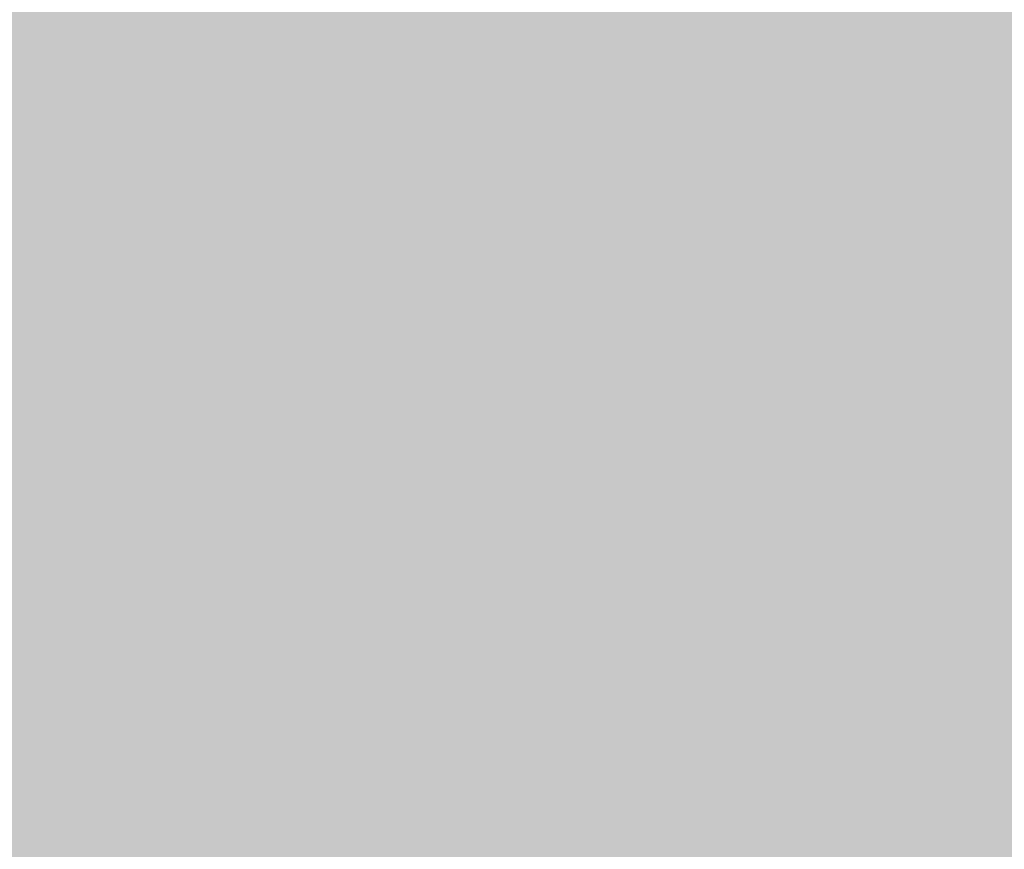
# Model space of a CAD drawing. Units: feet. Extents: x 3168 to 4724, y 827 to 1477.
# Tile 55 of 256: x 3273.13944 to 3273.15625, y 1099.00068 to 1099.01485. Entities that reach past the tile are written whole.
import ezdxf

# ---------------------------------------------------------------- set-up
doc = ezdxf.new("R2010")
doc.units = ezdxf.units.FT
doc.layers.add('A-ELEV', color=7, linetype='Continuous', lineweight=35)
doc.layers.add('A-ELEV-PATT', color=8, linetype='Continuous', lineweight=13)

msp = doc.modelspace()

# ---------------------------------------------------------------- hatches: boundary and pattern name
at = {"layer": 'A-ELEV-PATT'}
h = msp.add_hatch(color=256, dxfattribs=at)
h.dxf.hatch_style = 1
edge = h.paths.add_edge_path()
edge.add_ellipse((3552.905762, 979.220141), major_axis=(36.744924, 0), ratio=0.484848485, start_angle=0, end_angle=360)
edge = h.paths.add_edge_path()
edge.add_ellipse((3559.891637, 929.252282), major_axis=(36.744924, 0), ratio=0.484848485, start_angle=0, end_angle=360)
edge = h.paths.add_edge_path()
edge.add_line((3299.31681, 1198.606081), (3479.916714, 1198.606081))
edge.add_line((3479.916714, 1198.606081), (3479.916714, 1209.86857))
edge.add_spline(control_points=[(3479.916714, 1209.86857), (3464.301157, 1209.86857), (3448.685601, 1209.86857), (3410.949139, 1209.86857), (3388.828234, 1209.86857), (3355.646876, 1209.86857), (3344.586423, 1209.86857), (3327.995745, 1209.86857), (3322.465518, 1209.86857), (3314.170179, 1209.86857), (3311.405066, 1209.86857), (3307.257396, 1209.86857), (3305.874839, 1209.86857), (3303.801005, 1209.86857), (3303.109726, 1209.86857), (3302.072809, 1209.86857), (3301.72717, 1209.86857), (3301.208711, 1209.86857), (3301.035891, 1209.86857), (3300.776662, 1209.86857), (3300.690252, 1209.86857), (3300.560638, 1209.86857), (3300.517433, 1209.86857), (3300.452625, 1209.86857), (3300.431023, 1209.86857), (3300.398619, 1209.86857), (3300.387818, 1209.86857), (3300.366216, 1209.86857), (3300.345676, 1209.86857), (3300.345548, 1209.86857), (3300.345505, 1209.86857), (3300.343304, 1209.86857), (3300.341146, 1209.868571), (3300.337909, 1209.868571), (3300.33683, 1209.868572), (3300.333942, 1209.868573), (3300.332133, 1209.868574), (3300.325515, 1209.868577), (3300.320706, 1209.868581), (3300.310925, 1209.868592), (3300.305952, 1209.868598), (3300.290511, 1209.868623), (3300.280045, 1209.868646), (3300.232425, 1209.868777), (3300.195298, 1209.868954), (3299.951068, 1209.870608), (3299.744824, 1209.874326), (3299.436827, 1209.883257), (3299.334389, 1209.886792), (3299.181079, 1209.89292), (3299.130033, 1209.895099), (3298.652217, 1209.916801), (3298.22946, 1209.945718), (3297.601631, 1210.002367), (3297.393404, 1210.023464), (3297.082652, 1210.058309), (3296.979332, 1210.070458), (3296.292954, 1210.154861), (3295.718148, 1210.243356), (3294.868717, 1210.39885), (3294.5877, 1210.454478), (3294.169341, 1210.543349), (3294.030415, 1210.573878), (3291.707149, 1211.1012), (3289.65359, 1211.813435), (3285.776259, 1213.563988), (3283.95141, 1214.603478), (3280.512159, 1216.98008), (3278.897241, 1218.317592), (3276.379914, 1220.829489), (3275.416042, 1221.917738), (3274.039342, 1223.7077), (3273.581043, 1224.349535), (3273.143228, 1225.016316)], knot_values=[39.119033, 39.119033, 39.119033, 39.119033, 39.286353, 39.286353, 39.523379, 39.523379, 39.641892, 39.641892, 39.701148, 39.701148, 39.730777, 39.730777, 39.745591, 39.745591, 39.752998, 39.752998, 39.756701, 39.756701, 39.758553, 39.758553, 39.759479, 39.759479, 39.759942, 39.759942, 39.760173, 39.760173, 39.760289, 39.760289, 39.760405, 39.760405, 39.760463, 39.760463, 39.763389, 39.763389, 39.764851, 39.764851, 39.767304, 39.767304, 39.773825, 39.773825, 39.78057, 39.78057, 39.79477, 39.79477, 39.845194, 39.845194, 40.126715, 40.126715, 40.267476, 40.267476, 40.337856, 40.337856, 40.927023, 40.927023, 41.221606, 41.221606, 41.368898, 41.368898, 42.202622, 42.202622, 42.619485, 42.619485, 42.827916, 42.827916, 46.118323, 46.118323, 49.408731, 49.408731, 52.699139, 52.699139, 54.927489, 54.927489, 56.104228, 56.104228, 56.104228, 56.104228], weights=[1, 1, 1, 1, 1, 1, 1, 1, 1, 1, 1, 1, 1, 1, 1, 1, 1, 1, 1, 1, 1, 1, 1, 1, 1, 1, 1, 1, 1, 1, 1, 1, 1, 1, 1, 1, 1, 1, 1, 1, 1, 1, 1, 1, 1, 1, 1, 1, 1, 1, 1, 1, 1, 1, 1, 1, 1, 1, 1, 1, 1, 1, 1, 1, 1, 1, 1, 1, 1, 1, 1, 1, 1, 1], degree=3, periodic=0)
edge.add_line((3273.143228, 1225.016316), (3273.143228, 1099.016316))
edge.add_line((3273.143228, 1099.016316), (3299.31681, 1099.016316))
edge.add_line((3299.31681, 1099.016316), (3299.31681, 1198.606081))
edge = h.paths.add_edge_path()
edge.add_line((3304.758443, 1324.15806), (3479.916714, 1324.15806))
edge.add_line((3479.916714, 1324.15806), (3479.916714, 1335.714618))
edge.add_line((3479.916714, 1335.714618), (3269.161628, 1335.714618))
edge.add_spline(control_points=[(3269.161628, 1335.714618), (3264.024231, 1335.714618), (3258.364118, 1328.958189), (3259.264311, 1323.900274)], knot_values=[0, 0, 0, 0, 15.412191, 15.412191, 15.412191, 15.412191], degree=3, periodic=0)
edge.add_line((3259.264311, 1323.900274), (3265.516849, 1288.769135))
edge.add_line((3265.516849, 1288.769135), (3275.265103, 1261.545626))
edge.add_line((3275.265103, 1261.545626), (3304.758443, 1261.545626))
edge.add_line((3304.758443, 1261.545626), (3304.758443, 1324.15806))
h = msp.add_hatch(color=256, dxfattribs=at)
h.dxf.hatch_style = 1
h.paths.add_polyline_path([(3384.525247, 1099.016316), (3335.029168, 1099.016316), (3299.31681, 1099.016316), (3273.143228, 1099.016316), (3217.565364, 1099.016316), (3168.069285, 827.11626), (3335.029168, 827.11626)])

# ---------------------------------------------------------------- linework, layer by layer
at = {"layer": 'A-ELEV'}
msp.add_open_spline([(3808.5202, 1099.016316), (3808.5202, 1141.413235), (3808.5202, 1183.810154), (3808.5202, 1226.635324), (3808.5202, 1227.063576), (3808.5202, 1227.491828), (3811.491871, 1248.994673), (3814.463542, 1270.497518), (3817.46523, 1292.217564), (3817.495247, 1292.434764), (3817.525264, 1292.651964), (3817.572801, 1310.106748), (3817.620339, 1327.561532), (3817.667877, 1345.016316), (3817.667877, 1345.457962), (3817.667877, 1345.899608), (3817.667877, 1346.456047), (3817.667877, 1346.57084), (3817.667877, 1346.752887), (3817.667877, 1346.820142), (3817.667877, 1346.93487), (3817.667877, 1346.982345), (3817.667877, 1347.038587), (3817.667877, 1347.047356), (3817.667877, 1347.073661), (3817.667877, 1347.059303), (3817.667877, 1347.061545), (3817.667876, 1347.062667), (3817.667875, 1347.066031), (3817.667874, 1347.068274), (3817.66787, 1347.075001), (3817.667866, 1347.079486), (3817.667849, 1347.092937), (3817.667833, 1347.101902), (3817.667766, 1347.12879), (3817.667699, 1347.146705), (3817.667432, 1347.200421), (3817.667165, 1347.236192), (3817.6661, 1347.343385), (3817.665038, 1347.414686), (3817.660812, 1347.628095), (3817.656608, 1347.769708), (3817.63997, 1348.192487), (3817.623509, 1348.471586), (3817.559094, 1349.300067), (3817.496121, 1349.840588), (3817.255432, 1351.424156), (3817.026318, 1352.428785), (3816.306871, 1354.888914), (3815.743745, 1356.268727), (3814.463959, 1358.81921), (3813.746413, 1359.990968), (3812.195838, 1362.172343), (3811.362245, 1363.182124), (3809.588836, 1365.069009), (3808.648816, 1365.946105), (3806.654262, 1367.579616), (3805.599702, 1368.336154), (3803.352891, 1369.722327), (3802.160535, 1370.352386), (3799.600813, 1371.453586), (3798.232688, 1371.925481), (3795.280084, 1372.634624), (3793.693148, 1372.872068), (3791.869441, 1372.92648), (3791.740861, 1372.92922), (3791.353371, 1372.934101), (3791.092707, 1372.932901), (3790.304116, 1372.915068), (3789.769543, 1372.884195), (3789.20919, 1372.830236), (3789.190622, 1372.828424), (3789.134892, 1372.822912), (3789.097705, 1372.819137), (3789.048445, 1372.814008), (3789.0364, 1372.812743), (3789.000256, 1372.808918), (3788.976147, 1372.806325), (3788.949405, 1372.803404), (3788.946786, 1372.803118), (3788.942567, 1372.802655), (3788.940967, 1372.80248), (3788.938572, 1372.802217), (3788.937777, 1372.802129), (3788.935391, 1372.801867), (3788.867535, 1372.794402), (3788.756866, 1372.782228), (3788.701532, 1372.776141), (3788.53553, 1372.75788), (3788.424861, 1372.745707), (3788.092856, 1372.709185), (3787.871519, 1372.684837), (3787.207509, 1372.611793), (3786.764835, 1372.563097), (3785.436814, 1372.417009), (3784.551467, 1372.319617), (3781.895425, 1372.027442), (3780.12473, 1371.832658), (3774.812646, 1371.248307), (3771.271256, 1370.858739), (3760.647088, 1369.690037), (3753.56431, 1368.910902), (3732.315973, 1366.573498), (3718.150416, 1365.015228), (3694.006758, 1362.359326), (3684.028657, 1361.261694), (3674.050557, 1360.164062), (3664.600662, 1360.164062), (3655.150767, 1360.164062), (3626.801081, 1360.164062), (3607.901291, 1360.164062), (3551.20192, 1360.164062), (3513.40234, 1360.164062), (3467.725182, 1360.164062), (3459.847604, 1360.164062), (3436.214873, 1360.164062), (3420.459718, 1360.164062), (3373.194255, 1360.164062), (3341.683946, 1360.164062), (3302.848162, 1360.164062), (3295.522686, 1360.164062), (3286.038292, 1360.164062), (3283.879372, 1360.164062), (3277.402613, 1360.164062), (3273.084773, 1360.164062), (3267.732851, 1360.164062), (3266.698768, 1360.164062), (3263.59652, 1360.164062), (3261.528355, 1360.164062), (3259.236943, 1360.164062), (3259.013697, 1360.164062), (3258.343958, 1360.164062), (3257.897466, 1360.164062), (3257.430998, 1360.164062), (3257.411022, 1360.164062), (3257.370573, 1360.164062), (3257.37547, 1360.164062), (3257.374598, 1360.164062), (3257.373937, 1360.164062), (3257.371956, 1360.164062), (3257.370635, 1360.164061), (3257.366673, 1360.16406), (3257.364032, 1360.164059), (3257.356109, 1360.164053), (3257.350828, 1360.164047), (3257.334987, 1360.164023), (3257.32443, 1360.163998), (3257.292769, 1360.163899), (3257.271676, 1360.163799), (3257.208439, 1360.163398), (3257.166337, 1360.162995), (3257.040206, 1360.161388), (3256.956349, 1360.159783), (3256.705504, 1360.153393), (3256.53924, 1360.147036), (3256.04357, 1360.121916), (3255.717296, 1360.097102), (3254.752446, 1360.000481), (3254.127968, 1359.906513), (3252.180067, 1359.525332), (3250.941574, 1359.143991), (3248.670175, 1358.24329), (3247.635739, 1357.723834), (3245.732632, 1356.603471), (3244.863388, 1356.00206), (3243.253108, 1354.742865), (3242.511972, 1354.084731), (3240.751052, 1352.344781), (3239.800961, 1351.229574), (3238.087769, 1348.87244), (3237.324685, 1347.630355), (3235.98251, 1344.971632), (3235.402205, 1343.554907), (3234.591081, 1340.815458), (3234.310882, 1339.54355), (3233.97649, 1336.802561), (3233.922113, 1335.330877), (3234.148916, 1332.591269), (3234.349529, 1331.367201), (3234.719893, 1329.999367), (3234.752423, 1329.883362), (3234.853619, 1329.534797), (3234.925892, 1329.301685), (3235.024836, 1329.002552), (3235.046924, 1328.936928), (3235.077639, 1328.847239), (3235.085924, 1328.823198), (3235.110939, 1328.751064), (3235.127828, 1328.702962), (3235.147992, 1328.646242), (3235.151059, 1328.637632), (3235.156096, 1328.623526), (3235.158061, 1328.61803), (3235.160209, 1328.61203), (3235.165612, 1328.596943), (3235.180099, 1328.556486), (3235.190263, 1328.528101), (3235.220756, 1328.442946), (3235.241084, 1328.386176), (3235.302069, 1328.215865), (3235.342726, 1328.102325), (3235.464696, 1327.761704), (3235.54601, 1327.534623), (3235.78995, 1326.853381), (3235.952577, 1326.39922), (3236.440459, 1325.036736), (3236.765713, 1324.128414), (3237.741475, 1321.403446), (3238.391983, 1319.586801), (3240.343508, 1314.136866), (3241.644525, 1310.503576), (3245.547574, 1299.603706), (3248.149607, 1292.337126), (3255.955706, 1270.537385), (3261.159772, 1256.004225), (3267.387618, 1238.612001), (3268.411397, 1235.752937), (3269.510378, 1232.683864), (3269.585579, 1232.473854), (3269.706612, 1232.135851), (3269.752444, 1232.007857), (3269.827329, 1231.79873), (3269.856382, 1231.717595), (3269.906325, 1231.578122), (3269.927215, 1231.519782), (3269.972468, 1231.393406), (3269.996831, 1231.325368), (3270.026503, 1231.242506), (3270.031811, 1231.227681), (3270.040282, 1231.204024), (3270.039224, 1231.206979), (3270.039359, 1231.206601), (3270.039427, 1231.206412), (3270.03963, 1231.205846), (3270.039765, 1231.205468), (3270.040171, 1231.204335), (3270.040442, 1231.203579), (3270.041254, 1231.201313), (3270.041796, 1231.199802), (3270.04342, 1231.195269), (3270.044504, 1231.192248), (3270.047756, 1231.183185), (3270.049926, 1231.177145), (3270.056442, 1231.159028), (3270.060793, 1231.146957), (3270.073867, 1231.110761), (3270.082613, 1231.086656), (3270.108936, 1231.014413), (3270.1266, 1230.96635), (3270.179934, 1230.822457), (3270.215947, 1230.726923), (3270.325323, 1230.441508), (3270.400026, 1230.252811), (3270.629249, 1229.691444), (3270.788883, 1229.323501), (3271.286488, 1228.238319), (3271.6431, 1227.539755), (3272.775859, 1225.515277), (3273.614169, 1224.260502), (3275.416042, 1221.917738), (3276.379914, 1220.829489), (3278.897241, 1218.317592), (3280.512159, 1216.98008), (3283.95141, 1214.603478), (3285.776259, 1213.563988), (3289.65359, 1211.813435), (3291.707149, 1211.1012), (3294.030415, 1210.573878), (3294.169341, 1210.543349), (3294.5877, 1210.454478), (3294.868717, 1210.39885), (3295.718148, 1210.243356), (3296.292954, 1210.154861), (3296.979332, 1210.070458), (3297.082652, 1210.058309), (3297.393404, 1210.023464), (3297.601631, 1210.002367), (3298.22946, 1209.945718), (3298.652217, 1209.916801), (3299.130033, 1209.895099), (3299.181079, 1209.89292), (3299.334389, 1209.886792), (3299.436827, 1209.883257), (3299.744824, 1209.874326), (3299.951068, 1209.870608), (3300.195298, 1209.868954), (3300.232425, 1209.868777), (3300.280045, 1209.868646), (3300.290511, 1209.868623), (3300.305952, 1209.868598), (3300.310925, 1209.868592), (3300.320706, 1209.868581), (3300.325515, 1209.868577), (3300.332133, 1209.868574), (3300.333942, 1209.868573), (3300.33683, 1209.868572), (3300.337909, 1209.868571), (3300.341146, 1209.868571), (3300.343304, 1209.86857), (3300.345505, 1209.86857), (3300.345548, 1209.86857), (3300.345676, 1209.86857), (3300.366216, 1209.86857), (3300.387818, 1209.86857), (3300.398619, 1209.86857), (3300.431023, 1209.86857), (3300.452625, 1209.86857), (3300.517433, 1209.86857), (3300.560638, 1209.86857), (3300.690252, 1209.86857), (3300.776662, 1209.86857), (3301.035891, 1209.86857), (3301.208711, 1209.86857), (3301.72717, 1209.86857), (3302.072809, 1209.86857), (3303.109726, 1209.86857), (3303.801005, 1209.86857), (3305.874839, 1209.86857), (3307.257396, 1209.86857), (3311.405066, 1209.86857), (3314.170179, 1209.86857), (3322.465518, 1209.86857), (3327.995745, 1209.86857), (3344.586423, 1209.86857), (3355.646876, 1209.86857), (3388.828234, 1209.86857), (3410.949139, 1209.86857), (3477.311855, 1209.86857), (3521.553665, 1209.86857), (3566.836184, 1209.86857), (3567.876892, 1209.86857), (3570.999017, 1209.86857), (3573.080433, 1209.86857), (3575.781396, 1209.86857), (3576.400943, 1209.86857), (3577.295821, 1209.86857), (3577.571152, 1209.86857), (3578.397146, 1209.86857), (3578.947808, 1209.86857), (3579.756491, 1209.86857), (3580.014511, 1209.86857), (3580.342737, 1209.86857), (3580.326865, 1209.86857), (3580.32717, 1209.86857), (3580.327323, 1209.86857), (3580.327781, 1209.86857), (3580.328086, 1209.86857), (3580.329002, 1209.86857), (3580.329613, 1209.86857), (3580.331445, 1209.86857), (3580.332667, 1209.86857), (3580.336332, 1209.868569), (3580.338775, 1209.868567), (3580.346107, 1209.868563), (3580.350995, 1209.868558), (3580.365663, 1209.86854), (3580.375445, 1209.868522), (3580.404801, 1209.868449), (3580.424386, 1209.868376), (3580.483183, 1209.868085), (3580.522437, 1209.867793), (3580.640361, 1209.866624), (3580.719195, 1209.865454), (3580.956315, 1209.860766), (3581.115222, 1209.85607), (3581.594164, 1209.83723), (3581.916419, 1209.818331), (3582.889947, 1209.742428), (3583.547986, 1209.666169), (3585.531827, 1209.360617), (3586.867216, 1209.053886), (3589.471545, 1208.252472), (3590.740241, 1207.757852), (3591.995451, 1207.158802), (3592.057809, 1207.12874), (3592.244242, 1207.037954), (3592.367676, 1206.976632), (3592.73528, 1206.790359), (3592.976752, 1206.663101), (3593.244539, 1206.516441), (3593.274731, 1206.499825), (3593.365115, 1206.449839), (3593.425113, 1206.416333), (3593.604314, 1206.315285), (3593.722725, 1206.247211), (3593.857212, 1206.168398), (3593.874362, 1206.158319), (3593.925741, 1206.128041), (3593.959899, 1206.107798), (3594.062086, 1206.046899), (3594.129827, 1206.006074), (3594.208436, 1205.958171), (3594.219683, 1205.951304), (3594.253391, 1205.930686), (3594.275819, 1205.916917), (3594.342972, 1205.875536), (3594.387563, 1205.847853), (3594.433616, 1205.81905), (3594.435256, 1205.818024), (3594.440175, 1205.814946), (3594.443453, 1205.812894), (3594.447123, 1205.810594), (3594.447516, 1205.810348), (3594.448695, 1205.80961), (3594.449481, 1205.809117), (3594.450366, 1205.808562), (3594.450466, 1205.8085), (3594.4506, 1205.808415), (3594.467399, 1205.797887), (3594.493269, 1205.781674), (3594.506204, 1205.773568), (3594.545008, 1205.749248), (3594.570878, 1205.733035), (3594.648487, 1205.684396), (3594.700226, 1205.651969), (3594.855444, 1205.554691), (3594.958922, 1205.489839), (3595.269357, 1205.295282), (3595.476314, 1205.165577), (3596.097185, 1204.776463), (3596.511099, 1204.517054), (3597.752841, 1203.738826), (3598.580669, 1203.220007), (3601.064152, 1201.663551), (3602.719807, 1200.625914), (3607.686774, 1197.513002), (3610.998085, 1195.437727), (3620.932018, 1189.211903), (3627.55464, 1185.061354), (3647.422507, 1172.609707), (3660.667751, 1164.308608), (3700.403484, 1139.405313), (3726.893973, 1122.803116), (3757.205715, 1103.806052), (3761.02697, 1101.411184), (3764.848224, 1099.016316), (3745.328271, 1099.016316), (3725.808319, 1099.016316), (3706.288366, 1099.016316), (3706.288366, 1108.453237), (3706.288366, 1117.890158), (3706.288366, 1127.327079), (3710.750754, 1127.327079), (3715.213143, 1127.327079), (3719.675531, 1127.327079)], degree=3, knots=[0, 0, 0, 0, 0.982037, 0.982037, 0.991957, 0.991957, 0.991957, 1.966522, 1.966522, 1.976367, 1.976367, 1.976367, 2.976367, 2.976367, 2.976367, 3.00169, 3.00169, 3.008272, 3.008272, 3.012129, 3.012129, 3.014851, 3.014851, 3.015353, 3.015353, 3.016359, 3.016359, 3.017365, 3.017365, 3.019376, 3.019376, 3.023398, 3.023398, 3.031442, 3.031442, 3.047531, 3.047531, 3.079708, 3.079708, 3.144063, 3.144063, 3.272772, 3.272772, 3.53019, 3.53019, 4.045026, 4.045026, 5.074698, 5.074698, 6.700878, 6.700878, 8.327058, 8.327058, 9.953238, 9.953238, 11.579418, 11.579418, 13.205598, 13.205598, 14.831778, 14.831778, 16.457958, 16.457958, 18.084138, 18.084138, 18.206872, 18.206872, 18.45234, 18.45234, 18.943275, 18.943275, 18.960093, 18.960093, 18.993729, 18.993729, 19.00461, 19.00461, 19.026374, 19.026374, 19.028737, 19.028737, 19.03018, 19.03018, 19.030897, 19.030897, 19.032332, 19.032332, 19.033766, 19.033766, 19.036636, 19.036636, 19.042374, 19.042374, 19.053851, 19.053851, 19.076805, 19.076805, 19.122714, 19.122714, 19.21453, 19.21453, 19.398163, 19.398163, 19.765429, 19.765429, 20.024128, 20.024128, 20.024128, 20.092031, 20.092031, 20.227836, 20.227836, 20.499446, 20.499446, 20.556051, 20.556051, 20.66926, 20.66926, 20.895678, 20.895678, 20.948316, 20.948316, 20.963829, 20.963829, 20.994855, 20.994855, 21.002285, 21.002285, 21.017146, 21.017146, 21.01875, 21.01875, 21.021959, 21.021959, 21.022102, 21.022102, 21.022249, 21.022249, 21.022708, 21.022708, 21.023627, 21.023627, 21.025464, 21.025464, 21.029138, 21.029138, 21.036486, 21.036486, 21.051183, 21.051183, 21.080575, 21.080575, 21.139361, 21.139361, 21.256932, 21.256932, 21.492073, 21.492073, 21.962356, 21.962356, 23.01002, 23.01002, 24.057684, 24.057684, 25.105348, 25.105348, 26.153011, 26.153011, 27.776787, 27.776787, 29.400562, 29.400562, 31.024337, 31.024337, 32.278801, 32.278801, 33.533265, 33.533265, 34.467568, 34.467568, 34.553971, 34.553971, 34.726776, 34.726776, 34.775309, 34.775309, 34.793079, 34.793079, 34.82862, 34.82862, 34.834979, 34.834979, 34.839039, 34.839039, 34.839411, 34.839411, 34.840285, 34.840285, 34.842034, 34.842034, 34.845531, 34.845531, 34.852525, 34.852525, 34.866512, 34.866512, 34.894488, 34.894488, 34.950439, 34.950439, 35.062342, 35.062342, 35.286147, 35.286147, 35.733758, 35.733758, 35.821815, 35.821815, 35.828283, 35.828283, 35.832225, 35.832225, 35.834724, 35.834724, 35.836521, 35.836521, 35.838617, 35.838617, 35.839073, 35.839073, 35.839345, 35.839345, 35.839617, 35.839617, 35.840161, 35.840161, 35.841249, 35.841249, 35.843425, 35.843425, 35.847778, 35.847778, 35.856482, 35.856482, 35.873891, 35.873891, 35.908709, 35.908709, 35.978345, 35.978345, 36.117617, 36.117617, 36.396161, 36.396161, 36.953248, 36.953248, 38.067423, 38.067423, 40.295772, 40.295772, 42.524122, 42.524122, 45.81453, 45.81453, 49.104937, 49.104937, 52.395345, 52.395345, 52.603776, 52.603776, 53.020639, 53.020639, 53.854363, 53.854363, 54.001655, 54.001655, 54.296238, 54.296238, 54.885405, 54.885405, 54.955785, 54.955785, 55.096546, 55.096546, 55.378067, 55.378067, 55.42849, 55.42849, 55.442691, 55.442691, 55.449436, 55.449436, 55.455957, 55.455957, 55.458409, 55.458409, 55.459872, 55.459872, 55.462798, 55.462798, 55.462856, 55.462856, 55.462972, 55.462972, 55.463088, 55.463088, 55.463319, 55.463319, 55.463782, 55.463782, 55.464708, 55.464708, 55.46656, 55.46656, 55.470263, 55.470263, 55.47767, 55.47767, 55.492484, 55.492484, 55.522112, 55.522112, 55.581369, 55.581369, 55.699882, 55.699882, 55.936907, 55.936907, 56.410959, 56.410959, 56.42211, 56.42211, 56.444413, 56.444413, 56.451051, 56.451051, 56.454001, 56.454001, 56.459901, 56.459901, 56.462666, 56.462666, 56.463418, 56.463418, 56.464171, 56.464171, 56.465675, 56.465675, 56.468684, 56.468684, 56.474702, 56.474702, 56.486738, 56.486738, 56.51081, 56.51081, 56.558955, 56.558955, 56.655243, 56.655243, 56.847821, 56.847821, 57.232975, 57.232975, 58.003284, 58.003284, 59.543901, 59.543901, 62.625137, 62.625137, 68.787607, 68.787607, 74.950078, 74.950078, 75.27336, 75.27336, 75.919923, 75.919923, 77.213051, 77.213051, 77.377769, 77.377769, 77.707206, 77.707206, 78.366079, 78.366079, 78.462532, 78.462532, 78.655436, 78.655436, 79.041245, 79.041245, 79.105735, 79.105735, 79.234714, 79.234714, 79.492672, 79.492672, 79.502197, 79.502197, 79.521249, 79.521249, 79.523534, 79.523534, 79.528103, 79.528103, 79.528682, 79.528682, 79.528885, 79.528885, 79.529089, 79.529089, 79.529495, 79.529495, 79.530308, 79.530308, 79.531935, 79.531935, 79.535187, 79.535187, 79.541693, 79.541693, 79.554704, 79.554704, 79.580725, 79.580725, 79.632769, 79.632769, 79.736856, 79.736856, 79.94503, 79.94503, 80.361377, 80.361377, 80.421435, 80.421435, 80.421435, 81.421435, 81.421435, 81.421435, 82.421435, 82.421435, 82.421435, 83.421435, 83.421435, 83.421435, 83.421435], dxfattribs=at)

doc.saveas('drawing.dxf')
